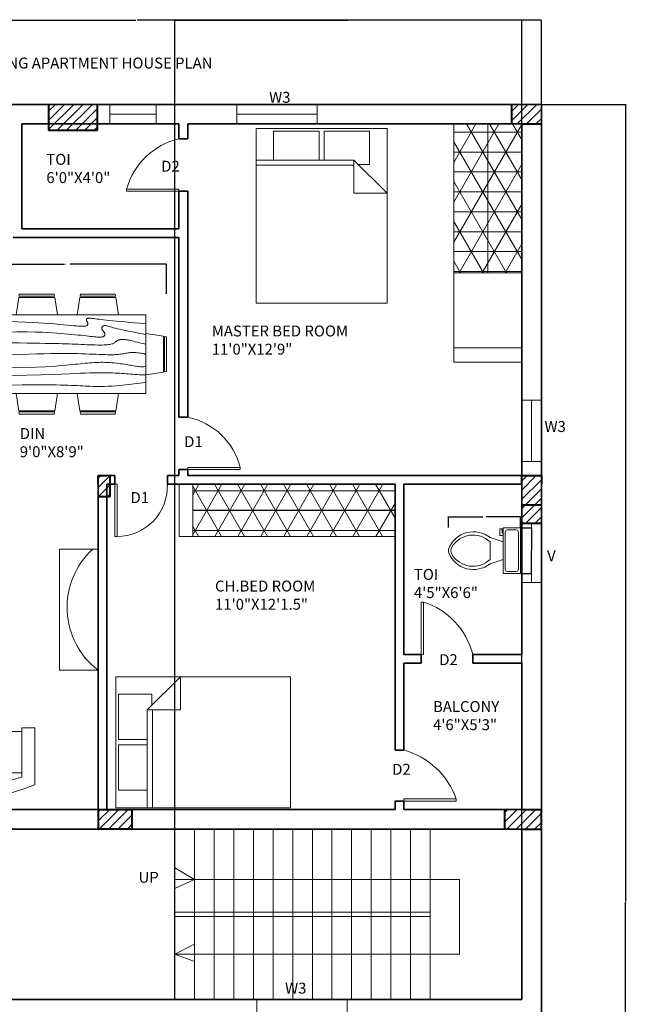
# Model space of a CAD drawing. Units: inches. Extents: x -86 to 2463, y -1058 to 68.
# Tile 17 of 17: x 148 to 426, y -383 to 68. Entities that reach past the tile are written whole.
import ezdxf

# ---------------------------------------------------------------- set-up
doc = ezdxf.new("R2010")
doc.units = ezdxf.units.IN
doc.header["$MEASUREMENT"] = 0
for name, color, linetype, lineweight in [('A-ANNO-DIMS', 2, 'Continuous', 18), ('A-ANNO-TEXT', 7, 'Continuous', 18), ('A-ANNO-TITL', 7, 'Continuous', 25), ('A-AREA-IDEN', 7, 'Continuous', 18), ('A-COLS', 7, 'Continuous', 40), ('A-COLS-PATT', 252, 'Continuous', 13), ('A-DOOR', 3, 'Continuous', 18), ('A-FLOR-CASE', 8, 'Continuous', 18), ('A-FLOR-CASE-PATT', 252, 'Continuous', 13), ('A-FLOR-FIXT', 9, 'Continuous', 18), ('A-FLOR-STRS', 7, 'Continuous', 18), ('A-FURN', 8, 'Continuous', 18), ('A-GLAZ', 4, 'Continuous', 18), ('A-WALL', 7, 'Continuous', 35)]:
    doc.layers.add(name, color=color, linetype=linetype, lineweight=lineweight)
doc.styles.get("Standard").update_dxf_attribs({"font": 'arial.ttf'})
doc.dimstyles.get("Standard").update_dxf_attribs({"dimtxt": 0.18, "dimasz": 0.18, "dimexe": 0.18, "dimexo": 0.0625, "dimgap": 0.09, "dimtad": 0, "dimtih": 1, "dimtoh": 1, "dimdec": 4, "dimzin": 0, "dimdsep": 46, "dimtxsty": 'Standard', "dimcen": 0.09, "dimadec": 0, "dimazin": 0, "dimtfac": 1, "dimtdec": 4, "dimtofl": 0, "dimtmove": 0, "dimatfit": 3, "dimfxl": 1, "dimtolj": 1, "dimtzin": 0, "dimarcsym": 0})
pattern_1 = [(45, (-1015.1314, -586.0864), (-2.1213203, 2.1213203), [])]
pattern_2 = [(0, (-1015.131, -586.086), (0, 9.125), []), (60, (-1015.131, -586.086), (-7.90248, 4.5625), []), (120, (-1015.131, -586.086), (-7.90248, -4.5625), [])]

# ---------------------------------------------------------------- blocks, each defined once
blk = doc.blocks.new('Bed - Queen')
for p, q in [((0, -80.00003), (0, 0)), ((0, 0), (59.99999, 0)), ((59.99999, 0), (59.99999, -80.00003)), ((7.99999, -1.2), (28.79998, -1.2)), ((7.99999, -14.4), (7.99999, -1.2)), ((28.79998, -1.2), (28.79998, -14.4)), ((31.19999, -1.2), (51.99999, -1.2)), ((31.19999, -14.4), (31.19999, -1.2)), ((51.99999, -1.2), (51.99999, -16.4)), ((0, -14.4), (44.8, -14.4)), ((44.8, -16.8), (0, -16.8)), ((59.99999, -29.6), (44.8, -14.4)), ((44.8, -14.4), (44.8, -29.6)), ((51.99999, -16.4), (46.79936, -16.4)), ((44.8, -29.6), (59.99999, -29.6)), ((59.99999, -80.00003), (0, -80.00003))]:
    blk.add_line(p, q)
blk = doc.blocks.new('Toilet - top')
for p, q in [((9.5, -6), (9.5, -2)), ((-10, -8.5), (-8, -8.5)), ((-10, -9.5), (-10, -8.5)), ((-8, -8.5), (-8, -8)), ((-7, -8), (-7, -9.5)), ((-4, -8), (-6, -14)), ((4, -8), (6, -14)), ((-7, -9.5), (-10, -9.5)), ((4, -14), (-4, -14))]:
    blk.add_line(p, q)
blk.add_lwpolyline([(10.5, -8), (10.5, 0), (-10.5, 0), (-10.5, -8)], close=True)
for points in [[(-9.5, -2), (-9.5, -6)], [(8.5, -1), (-8.5, -1)], [(-8.5, -7), (8.5, -7)]]:
    blk.add_lwpolyline(points)
for centre, radius, start, end in [((-8.62, -1.88), 0.884, 81.8699, 188.1301), ((8.62, -1.88), 0.884, 351.8699, 98.1301), ((-8.62, -6.12), 0.884, 171.8699, 278.1301), ((8.62, -6.12), 0.884, 261.8699, 8.1301), ((3.52, -21.58), 12.17, 141.4691, 247.9714), ((4.2, -21.82), 11.33, 136.3677, 238.9468), ((-3.52, -21.58), 12.17, 292.0284, 38.5307), ((-4.2, -21.82), 11.33, 301.053, 43.6321), ((0, -27.88), 4, 245.7318, 294.2682), ((0, -29), 4, 254.8605, 285.1395)]:
    blk.add_arc(centre, radius, start, end)
blk = doc.blocks.new('Sofa - Roundback 7 ft.')
for p, q in [((-12.00002, -32.4421), (-12.00003, -6.5971)), ((11.99997, -32.4421), (11.99998, -6.5971)), ((-36.000027, -34), (-36.000027, -11.4696)), ((-35.999844, -13.3819), (35.9998, -13.3819)), ((35.99998, -34), (35.99998, -11.4696)), ((-36.000027, -32.4421), (35.99998, -32.4421))]:
    blk.add_line(p, q)
for points in [[(-36.000027, -34), (-42.000027, -34), (-42.000027, -8)], [(41.99998, -8), (41.99998, -34), (35.99998, -34)]]:
    blk.add_lwpolyline(points)
for centre, radius, start, end in [((0, -114.25), 114.25, 68.43141, 111.5686), ((-0.00001, -127.1968), 121.1968, 72.72033, 107.2797)]:
    blk.add_arc(centre, radius, start, end)
blk = doc.blocks.new('Dining Set - 36 x 72 in.')
for p, q in [((-22, 27.5), (-22.1562, 26.50042)), ((-22, 27.5), (-6, 27.5)), ((-5.8437, 26.49966), (-6, 27.5)), ((6, 27.5), (5.8438, 26.50042)), ((6, 27.5), (22, 27.5)), ((22.1563, 26.49966), (22, 27.5)), ((-22.2343, 26.00059), (-23.4847, 17.99762)), ((-22.2304, 26), (-5.7608, 26)), ((-5.8416, 26.5), (-22.1534, 26.5)), ((-4.5152, 17.99762), (-5.7655, 25.99926)), ((5.7657, 26.00059), (4.5153, 17.99762)), ((5.7696, 26), (22.2392, 26)), ((22.1584, 26.5), (5.8466, 26.5)), ((23.4848, 17.99762), (22.2345, 25.99926)), ((36, 18), (-36, 18)), ((-36, 18), (-36, -18)), ((36, -18), (36, 18)), ((-44.0006, 8.23428), (-35.9976, 9.48474)), ((44.0006, 8.23428), (35.9976, 9.48474)), ((-45.5, 8), (-44.5004, 8.15617)), ((-45.5, 8), (-45.5, -8)), ((-44.5, -8.15843), (-44.5, 8.15338)), ((-44, 8.23041), (-44, -8.23915)), ((44, 8.23041), (44, -8.23915)), ((44.5, -8.15843), (44.5, 8.15338)), ((45.5, 8), (44.5005, 8.15617)), ((45.5, 8), (45.5, -8)), ((-44.4997, -8.15631), (-45.5, -8)), ((-35.9976, -9.48476), (-43.9993, -8.2345)), ((35.9976, -9.48476), (43.9993, -8.2345)), ((44.4997, -8.15631), (45.5, -8)), ((-36, -18), (36, -18)), ((-22.2343, -26.0006), (-23.4847, -17.99762)), ((-4.5152, -17.99762), (-5.7655, -25.99928)), ((5.7657, -26.0006), (4.5153, -17.99762)), ((23.4848, -17.99762), (22.2345, -25.99928)), ((-22.2304, -26), (-5.7608, -26)), ((-22, -27.5), (-22.1562, -26.50044)), ((-5.8416, -26.5), (-22.1534, -26.5)), ((-5.8437, -26.49967), (-6, -27.5)), ((5.7696, -26), (22.2392, -26)), ((6, -27.5), (5.8438, -26.50044)), ((22.1584, -26.5), (5.8466, -26.5)), ((22.1563, -26.49967), (22, -27.5)), ((-22, -27.5), (-6, -27.5)), ((6, -27.5), (22, -27.5))]:
    blk.add_line(p, q)
for points in [[(-36, 15), (-31.1772, 14.97754), (-26.8079, 14.91406), (-22.8538, 14.81543), (-19.276, 14.6875), (-16.0362, 14.53613), (-13.0957, 14.36718), (-10.4159, 14.18652), (-7.9583, 14), (-5.6904, 13.81315), (-3.6035, 13.63021), (-1.6954, 13.45508), (0.0365, 13.29166), (1.5945, 13.14388), (2.9811, 13.01562), (4.1988, 12.9108), (5.25, 12.83333), (6.1393, 12.78613), (6.8802, 12.76823), (7.4883, 12.77767), (7.9792, 12.8125), (8.3685, 12.87077), (8.6719, 12.95052), (8.9049, 13.0498), (9.0833, 13.16666), (9.2205, 13.29899), (9.3216, 13.44401), (9.3895, 13.59879), (9.4271, 13.76041), (9.4373, 13.92594), (9.4232, 14.09245), (9.3875, 14.257), (9.3333, 14.41666), (9.2638, 14.56917), (9.1836, 14.71484), (9.0975, 14.85465), (9.0104, 14.98958), (8.9272, 15.1206), (8.8529, 15.2487), (8.7922, 15.37483), (8.75, 15.5), (8.7305, 15.62467), (8.7344, 15.74739), (8.7617, 15.86621), (8.8125, 15.97916), (8.8867, 16.08431), (8.9844, 16.17968), (9.1055, 16.26334), (9.25, 16.33333), (9.4189, 16.38802), (9.6172, 16.42708), (9.8506, 16.45052), (10.125, 16.45833), (10.4463, 16.45052), (10.8203, 16.42708), (11.2529, 16.38802), (11.75, 16.33333), (12.3184, 16.26318), (12.9694, 16.17838), (13.7151, 16.07991), (14.5677, 15.96875), (15.5395, 15.84586), (16.6426, 15.71224), (17.8893, 15.56884), (19.2917, 15.41666), (20.859, 15.25667), (22.5879, 15.08984), (24.4721, 14.91715), (26.5052, 14.73958), (28.6809, 14.5581), (30.9929, 14.3737), (33.4347, 14.18733), (36, 14)], [(-36, 10), (-28.9766, 10.14274), (-23.1725, 10.20442), (-18.4241, 10.19775), (-14.5677, 10.13541), (-11.4399, 10.03011), (-8.877, 9.89453), (-6.7154, 9.74137), (-4.7917, 9.58333), (-2.9698, 9.43082), (-1.2246, 9.28515), (0.4415, 9.14534), (2.026, 9.01041), (3.5266, 8.87939), (4.9408, 8.7513), (6.266, 8.62516), (7.5, 8.5), (8.6411, 8.37549), (9.6914, 8.2539), (10.6538, 8.13818), (11.5312, 8.03125), (12.3267, 7.93603), (13.043, 7.85547), (13.6831, 7.79248), (14.25, 7.75), (14.7471, 7.7303), (15.1797, 7.73307), (15.5537, 7.75732), (15.875, 7.80208), (16.1494, 7.86637), (16.3828, 7.94922), (16.5811, 8.04964), (16.75, 8.16666), (16.8944, 8.29915), (17.0143, 8.44531), (17.1089, 8.60319), (17.1771, 8.77083), (17.218, 8.94629), (17.2305, 9.1276), (17.2137, 9.31282), (17.1667, 9.5), (17.0895, 9.6875), (16.987, 9.875), (16.8649, 10.0625), (16.7292, 10.25), (16.5856, 10.4375), (16.4401, 10.625), (16.2985, 10.8125), (16.1667, 11), (16.05, 11.18733), (15.9518, 11.3737), (15.8752, 11.5581), (15.8229, 11.73958), (15.798, 11.91715), (15.8034, 12.08984), (15.842, 12.25667), (15.9167, 12.41666), (16.0295, 12.56836), (16.1784, 12.70833), (16.3605, 12.83268), (16.5729, 12.9375), (16.8127, 13.01888), (17.0768, 13.07291), (17.3625, 13.0957), (17.6667, 13.08333), (17.9894, 13.03312), (18.3418, 12.94726), (18.7382, 12.82918), (19.1927, 12.68229), (19.7195, 12.51001), (20.3327, 12.31575), (21.0465, 12.10294), (21.875, 11.875), (22.8357, 11.63354), (23.959, 11.37304), (25.2786, 11.08618), (26.8282, 10.76562), (28.6414, 10.40405), (30.752, 9.99414), (33.1936, 9.52856), (36, 9)], [(-36, 5.5), (-30.7157, 5.3348), (-26.069, 5.20963), (-21.9946, 5.11767), (-18.4271, 5.05208), (-15.3009, 5.00602), (-12.5508, 4.97265), (-10.1112, 4.94515), (-7.9167, 4.91666), (-5.909, 4.88167), (-4.0586, 4.83984), (-2.3429, 4.79215), (-0.7396, 4.73958), (0.7739, 4.6831), (2.22, 4.6237), (3.6213, 4.56233), (5, 4.5), (6.373, 4.43782), (7.7344, 4.3776), (9.0723, 4.32129), (10.375, 4.27083), (11.6309, 4.22819), (12.8281, 4.19531), (13.9551, 4.17415), (15, 4.16666), (15.954, 4.17448), (16.819, 4.19791), (17.6001, 4.23698), (18.3021, 4.29166), (18.9299, 4.36198), (19.4883, 4.44791), (19.9823, 4.54948), (20.4167, 4.66666), (20.7969, 4.79899), (21.1302, 4.94401), (21.4245, 5.09879), (21.6875, 5.26041), (21.9271, 5.42594), (22.1511, 5.59245), (22.3672, 5.757), (22.5834, 5.91666), (22.8065, 6.06868), (23.0404, 6.21093), (23.2879, 6.34147), (23.5521, 6.45833), (23.8358, 6.55957), (24.142, 6.64323), (24.4735, 6.70735), (24.8334, 6.75), (25.2235, 6.76969), (25.642, 6.76692), (26.0858, 6.74267), (26.5521, 6.69791), (27.0379, 6.63362), (27.5404, 6.55078), (28.0565, 6.45036), (28.5834, 6.33333), (29.1242, 6.19987), (29.7071, 6.04687), (30.3661, 5.87044), (31.1354, 5.66666), (32.0493, 5.43164), (33.142, 5.16146), (34.4475, 4.85221), (36, 4.5)], [(-36, -1), (-30.7915, -0.6591), (-26.0195, -0.38216), (-21.6519, -0.16284), (-17.6563, 0.00521), (-14.0005, 0.12833), (-10.6523, 0.21289), (-7.5796, 0.26522), (-4.75, 0.29166), (-2.134, 0.29793), (0.2878, 0.28711), (2.5317, 0.26163), (4.6146, 0.22396), (6.5529, 0.17651), (8.3633, 0.12174), (10.0623, 0.06209), (11.6667, 0), (13.1899, -0.06201), (14.6341, -0.1211), (15.9982, -0.17432), (17.2813, -0.21875), (18.4823, -0.25147), (19.6003, -0.26953), (20.6343, -0.27002), (21.5834, -0.25), (22.4481, -0.20768), (23.2357, -0.14584), (23.9549, -0.06836), (24.6146, 0.02083), (25.2235, 0.11784), (25.7904, 0.21875), (26.3241, 0.31966), (26.8334, 0.41666), (27.3265, 0.50618), (27.8099, 0.58593), (28.2894, 0.65397), (28.7709, 0.70833), (29.2601, 0.74707), (29.763, 0.76823), (30.2855, 0.76985), (30.8334, 0.75), (31.4088, 0.70784), (31.9994, 0.64713), (32.589, 0.57275), (33.1615, 0.48958), (33.7008, 0.4025), (34.1908, 0.3164), (34.6153, 0.23616), (34.9584, 0.16666), (35.2099, 0.11165), (35.3848, 0.07031), (35.504, 0.04069), (35.5886, 0.02083), (35.6594, 0.00879), (35.7377, 0.0026), (35.8442, 0.00032), (36, 0)], [(-36, -6.5), (-27.1843, -6.31267), (-20.084, -6.1263), (-14.469, -5.9419), (-10.1094, -5.76042), (-6.7752, -5.58285), (-4.2363, -5.41016), (-2.2629, -5.24333), (-0.625, -5.08334), (0.8708, -4.93099), (2.2715, -4.78646), (3.5872, -4.64974), (4.8281, -4.52084), (6.0046, -4.39974), (7.127, -4.28646), (8.2053, -4.18099), (9.25, -4.08334), (10.2705, -3.99382), (11.2734, -3.91407), (12.2647, -3.84603), (13.25, -3.79167), (14.2354, -3.75293), (15.2266, -3.73177), (16.2295, -3.73015), (17.25, -3.75), (18.2912, -3.79248), (19.3451, -3.85547), (20.4009, -3.93604), (21.4479, -4.03125), (22.4754, -4.13819), (23.4727, -4.25391), (24.4289, -4.37549), (25.3334, -4.5), (26.1785, -4.62492), (26.9694, -4.74935), (27.7145, -4.87281), (28.4219, -4.99479), (29.1, -5.11483), (29.7572, -5.23242), (30.4016, -5.34709), (31.0417, -5.45834), (31.6837, -5.56437), (32.3262, -5.65821), (32.9658, -5.73153), (33.599, -5.77604), (34.2224, -5.78345), (34.8327, -5.74545), (35.4264, -5.65373), (36, -5.5)], [(-36, -10), (-26.4022, -9.81299), (-18.4675, -9.62891), (-11.9839, -9.45069), (-6.7396, -9.28125), (-2.5226, -9.12354), (0.8789, -8.98047), (3.6769, -8.85498), (6.0833, -8.75), (8.2767, -8.66765), (10.3021, -8.60677), (12.1712, -8.56543), (13.8958, -8.54167), (15.4876, -8.53353), (16.9583, -8.53907), (18.3197, -8.55632), (19.5834, -8.58334), (20.7616, -8.61841), (21.8685, -8.66081), (22.9188, -8.71004), (23.9271, -8.76563), (24.9081, -8.82707), (25.8763, -8.89388), (26.8465, -8.96558), (27.8334, -9.04167), (28.8474, -9.12118), (29.8828, -9.20117), (30.93, -9.27824), (31.9792, -9.34896), (33.0205, -9.40991), (34.0443, -9.45768), (35.0407, -9.48885), (36, -9.5)], [(-36, -14.5), (-30.0881, -14.33513), (-25.0332, -14.21224), (-20.7312, -14.12647), (-17.0781, -14.07292), (-13.97, -14.04671), (-11.3027, -14.04297), (-8.9724, -14.05681), (-6.875, -14.08334), (-4.9224, -14.11833), (-3.0905, -14.16016), (-1.3709, -14.20785), (0.2448, -14.26042), (1.7647, -14.3169), (3.1973, -14.3763), (4.5507, -14.43767), (5.8333, -14.5), (7.0554, -14.5621), (8.235, -14.62175), (9.3922, -14.67652), (10.5469, -14.72396), (11.7192, -14.76164), (12.929, -14.78711), (14.1965, -14.79794), (15.5417, -14.79167), (16.9933, -14.76424), (18.6152, -14.70508), (20.4804, -14.60197), (22.6615, -14.44271), (25.2312, -14.21509), (28.2624, -13.9069), (31.8277, -13.50594), (36, -13)]]:
    blk.add_lwpolyline(points)
blk = doc.blocks.new('DOOR-LEAF-24IN')
for p, q in [((0, 0), (0, 24)), ((0, 24), (1, 24)), ((1, 24), (1, 0)), ((1, 0), (0, 0))]:
    blk.add_line(p, q)
blk = doc.blocks.new('*D22')
at = {"layer": 'A-ANNO-DIMS', "color": 0, "lineweight": -2, "transparency": 16777216}
for p, q in [((344.18, -164.99), (344.18, -159.92)), ((344.36, -160.1), (359.93, -160.1)), ((377.05, -160.1), (361.48, -160.1)), ((377.23, -164.99), (377.23, -159.92))]:
    blk.add_line(p, q, dxfattribs=at)
at = {"layer": 'A-ANNO-DIMS', "color": 0, "transparency": 16777216}
for points in [[(344.36, -160.07), (344.36, -160.13), (344.18, -160.1)], [(377.05, -160.07), (377.05, -160.13), (377.23, -160.1)]]:
    blk.add_solid(points, dxfattribs=at)
at = {"layer": 'Defpoints', "color": 0, "transparency": 16777216}
for p in [(377.23, -160.1), (344.18, -165.05), (377.23, -165.05)]:
    blk.add_point(p, dxfattribs=at)
at = {"layer": 'A-ANNO-DIMS', "color": 0, "transparency": 16777216, "insert": (360.71, -160.1), "char_height": 0.18, "attachment_point": 5}
blk.add_mtext('\\A1;WC 33 TYP.', dxfattribs=at)
blk = doc.blocks.new('*D23')
at = {"layer": 'A-ANNO-DIMS', "color": 0, "lineweight": -2, "transparency": 16777216}
for p, q in [((377.29, -165.05), (382.37, -165.05)), ((382.19, -165.23), (382.19, -175.37)), ((382.19, -185.87), (382.19, -175.73)), ((377.29, -186.05), (382.37, -186.05))]:
    blk.add_line(p, q, dxfattribs=at)
at = {"layer": 'A-ANNO-DIMS', "color": 0, "transparency": 16777216}
for points in [[(382.16, -165.23), (382.22, -165.23), (382.19, -165.05)], [(382.16, -185.87), (382.22, -185.87), (382.19, -186.05)]]:
    blk.add_solid(points, dxfattribs=at)
at = {"layer": 'Defpoints', "color": 0, "transparency": 16777216}
for p in [(377.23, -165.05), (377.23, -186.05), (382.19, -186.05)]:
    blk.add_point(p, dxfattribs=at)
at = {"layer": 'A-ANNO-DIMS', "color": 0, "transparency": 16777216, "insert": (382.19, -175.55), "char_height": 0.18, "attachment_point": 5}
blk.add_mtext('\\A1;21 TYP.', dxfattribs=at)
blk = doc.blocks.new('*D28')
at = {"layer": 'A-ANNO-DIMS', "color": 0, "lineweight": -2, "transparency": 16777216}
for p, q in [((124.1, -57.97), (124.1, -44.2)), ((124.28, -44.38), (168.32, -44.38)), ((214.92, -44.38), (170.87, -44.38)), ((215.1, -57.97), (215.1, -44.2))]:
    blk.add_line(p, q, dxfattribs=at)
at = {"layer": 'A-ANNO-DIMS', "color": 0, "transparency": 16777216}
for points in [[(124.28, -44.35), (124.28, -44.41), (124.1, -44.38)], [(214.92, -44.35), (214.92, -44.41), (215.1, -44.38)]]:
    blk.add_solid(points, dxfattribs=at)
at = {"layer": 'Defpoints', "color": 0, "transparency": 16777216}
for p in [(215.1, -44.38), (124.1, -58.03), (215.1, -58.03)]:
    blk.add_point(p, dxfattribs=at)
at = {"layer": 'A-ANNO-DIMS', "color": 0, "transparency": 16777216, "insert": (169.6, -44.38), "char_height": 0.18, "attachment_point": 5}
blk.add_mtext('\\A1;DINING SET 91 TYP.', dxfattribs=at)
blk = doc.blocks.new('*D31')
at = {"layer": 'A-ANNO-DIMS', "color": 0, "lineweight": -2, "transparency": 16777216}
for p, q in [((386.82, 28.9), (425.54, 28.9)), ((425.36, 28.72), (425.36, -336.17)), ((425.36, -701.42), (425.36, -336.54)), ((386.82, -701.6), (425.54, -701.6))]:
    blk.add_line(p, q, dxfattribs=at)
at = {"layer": 'A-ANNO-DIMS', "color": 0, "transparency": 16777216}
for points in [[(425.33, 28.72), (425.39, 28.72), (425.36, 28.9)], [(425.33, -701.42), (425.39, -701.42), (425.36, -701.6)]]:
    blk.add_solid(points, dxfattribs=at)
at = {"layer": 'Defpoints', "color": 0, "transparency": 16777216}
for p in [(386.76, 28.9), (425.36, 28.9), (386.76, -701.6)]:
    blk.add_point(p, dxfattribs=at)
at = {"layer": 'A-ANNO-DIMS', "color": 0, "transparency": 16777216, "insert": (425.36, -336.35), "char_height": 0.18, "attachment_point": 5}
blk.add_mtext('\\A1;730.5', dxfattribs=at)
blk = doc.blocks.new('*D35')
at = {"layer": 'A-ANNO-DIMS', "color": 0, "lineweight": -2, "transparency": 16777216}
for p, q in [((15.76, 28.96), (15.76, 67.68)), ((386.76, 28.96), (386.76, 67.68)), ((15.94, 67.5), (200.99, 67.5)), ((386.58, 67.5), (201.53, 67.5))]:
    blk.add_line(p, q, dxfattribs=at)
at = {"layer": 'A-ANNO-DIMS', "color": 0, "transparency": 16777216}
for points in [[(15.94, 67.53), (15.94, 67.47), (15.76, 67.5)], [(386.58, 67.53), (386.58, 67.47), (386.76, 67.5)]]:
    blk.add_solid(points, dxfattribs=at)
at = {"layer": 'Defpoints', "color": 0, "transparency": 16777216}
for p in [(386.76, 67.5), (15.76, 28.9), (386.76, 28.9)]:
    blk.add_point(p, dxfattribs=at)
at = {"layer": 'A-ANNO-DIMS', "color": 0, "transparency": 16777216, "insert": (201.26, 67.5), "char_height": 0.18, "attachment_point": 5}
blk.add_mtext('\\A1;371', dxfattribs=at)
blk = doc.blocks.new('*D36')
at = {"layer": 'A-ANNO-DIMS', "color": 0, "lineweight": -2, "transparency": 16777216}
for p, q in [((218.85, -381.04), (218.85, 67.68)), ((377.85, -381.04), (377.85, 67.68)), ((219.03, 67.5), (298.07, 67.5)), ((377.67, 67.5), (298.63, 67.5))]:
    blk.add_line(p, q, dxfattribs=at)
at = {"layer": 'A-ANNO-DIMS', "color": 0, "transparency": 16777216}
for points in [[(219.03, 67.53), (219.03, 67.47), (218.85, 67.5)], [(377.67, 67.53), (377.67, 67.47), (377.85, 67.5)]]:
    blk.add_solid(points, dxfattribs=at)
at = {"layer": 'Defpoints', "color": 0, "transparency": 16777216}
for p in [(377.85, 67.5), (218.85, -381.1), (377.85, -381.1)]:
    blk.add_point(p, dxfattribs=at)
at = {"layer": 'A-ANNO-DIMS', "color": 0, "transparency": 16777216, "insert": (298.35, 67.5), "char_height": 0.18, "attachment_point": 5}
blk.add_mtext('\\A1;159', dxfattribs=at)

msp = doc.modelspace()

# ---------------------------------------------------------------- hatches: boundary and pattern name
at = {"layer": 'A-COLS-PATT'}
h = msp.add_hatch(dxfattribs=at)
h.set_pattern_fill('ANSI31', color=256, scale=24)
h.set_pattern_definition(pattern_1)
h.paths.add_polyline_path([(24.761, -294.104), (24.761, -284.978), (15.761, -284.978), (15.761, -303.104), (24.761, -303.104)])
h.paths.add_polyline_path([(199.1, -294.104), (183.761, -294.104), (183.761, -303.104), (199.1, -303.104)])
h.paths.add_polyline_path([(386.761, -294.104), (377.761, -294.104), (369.914, -294.104), (369.914, -303.104), (377.846, -303.104), (386.761, -303.104)])
h.paths.add_polyline_path([(386.761, -145.104), (386.761, -141.104), (377.761, -141.104), (377.761, -145.104), (377.761, -154.61), (386.761, -154.61)])
h.paths.add_polyline_path([(386.761, -154.61), (377.761, -154.61), (377.761, -162.891), (386.761, -162.891)])
h.paths.add_polyline_path([(24.761, -145.104), (24.761, -141.104), (15.761, -141.104), (15.761, -156.678), (24.761, -156.678)])
h.paths.add_polyline_path([(-38.239, 28.896), (-47.239, 28.896), (-47.239, 19.896), (-47.239, 12.652), (-38.239, 12.652), (-38.239, 19.896)])
h.paths.add_polyline_path([(24.761, 28.896), (15.761, 28.896), (15.761, 19.896), (15.761, 12.545), (24.761, 12.545), (24.761, 19.896)])
h.paths.add_polyline_path([(183.507, 19.896), (161.036, 19.896), (161.036, 17.001), (183.507, 17.001)])
h.paths.add_polyline_path([(183.507, 28.896), (161.036, 28.896), (161.036, 19.896), (183.507, 19.896)])
h.paths.add_polyline_path([(386.761, 28.896), (373.166, 28.896), (373.166, 19.896), (377.761, 19.896), (386.761, 19.896)])
h = msp.add_hatch(dxfattribs=at)
h.set_pattern_fill('ANSI31', color=256, scale=24)
h.set_pattern_definition(pattern_1)
h.paths.add_polyline_path([(189.136, -141.104), (187.761, -141.104), (183.761, -141.104), (183.761, -145.104), (183.761, -150.833), (187.761, -150.833), (187.761, -145.104), (189.136, -145.104)])
h.paths.add_polyline_path([(189.136, -145.104), (187.761, -145.104), (187.761, -150.833), (189.136, -150.833)], flags=17)
at = {"layer": 'A-FLOR-CASE-PATT'}
h = msp.add_hatch(dxfattribs=at)
h.set_pattern_fill('NET3', color=256, scale=73)
h.set_pattern_definition(pattern_2)
h.paths.add_polyline_path([(362.202, 19.896), (346.643, 19.896), (346.643, -48.262), (362.202, -48.262)])
h.paths.add_polyline_path([(377.761, 19.896), (362.202, 19.896), (362.202, -48.262), (377.761, -48.262)])
h.paths.add_polyline_path([(362.455, -390.104), (347.604, -390.104), (347.604, -460.245), (362.455, -460.245)])
h.paths.add_polyline_path([(377.846, -390.104), (362.455, -390.104), (362.455, -460.245), (377.846, -460.245), (377.846, -425.104), (377.846, -421.104)])
h = msp.add_hatch(dxfattribs=at)
h.set_pattern_fill('NET3', color=256, scale=73)
h.set_pattern_definition(pattern_2)
h.paths.add_polyline_path([(319.761, -145.104), (227.044, -145.104), (227.044, -157.07), (319.761, -157.07)])
h.paths.add_polyline_path([(319.761, -157.07), (227.044, -157.07), (227.044, -169.036), (319.761, -169.036)])
h.paths.add_polyline_path([(319.846, -547.104), (234.906, -547.104), (234.906, -563.554), (319.846, -563.554)])
h.paths.add_polyline_path([(319.846, -563.554), (234.906, -563.554), (234.906, -580.004), (319.846, -580.004)])

# ---------------------------------------------------------------- linework, layer by layer
at = {"layer": 'A-COLS'}
for p, q in [((161.036, 28.896), (161.036, 17.001)), ((183.507, 17.001), (183.507, 28.896)), ((373.166, 19.896), (373.166, 28.896)), ((377.761, 19.896), (386.761, 19.896)), ((161.036, 17.001), (183.507, 17.001)), ((183.761, -141.104), (187.761, -141.104)), ((183.761, -145.104), (183.761, -141.104)), ((189.136, -141.104), (189.136, -150.833)), ((377.761, -141.104), (386.761, -141.104)), ((377.761, -145.104), (377.761, -141.104)), ((386.761, -141.104), (386.761, -145.104)), ((189.136, -150.833), (183.761, -150.833)), ((377.761, -154.61), (386.761, -154.61)), ((377.761, -162.891), (386.761, -162.891)), ((183.761, -294.104), (199.1, -294.104)), ((183.761, -294.104), (183.761, -303.104)), ((199.1, -294.104), (199.1, -303.104)), ((369.914, -294.104), (369.914, -303.104)), ((377.761, -294.104), (386.761, -294.104)), ((386.761, -303.104), (386.761, -294.104)), ((199.1, -303.104), (183.488, -303.104)), ((377.846, -303.104), (386.761, -303.104))]:
    msp.add_line(p, q, dxfattribs=at)
at = {"layer": 'A-DOOR'}
msp.add_line((220.761, -9.914), (220.761, -9.914), dxfattribs=at)
for centre, radius, start, end in [((228.021, -18.512), 32.421, 102.9403, 164.62195), ((218.621, -144.874), 31.041, 13.84523, 78.59252), ((192.286, -145.928), 23.177, 270.40058, 2.03717), ((322.741, -231.116), 33.53, 13.82397, 72.69243), ((314.756, -300.701), 34.927, 19.09458, 75.05907)]:
    msp.add_arc(centre, radius, start, end, dxfattribs=at)
at = {"layer": 'A-FLOR-CASE'}
for p, q in [((346.643, -89.261), (346.643, 19.896)), ((362.202, -48.262), (362.202, 19.896)), ((346.643, -48.262), (377.761, -48.262)), ((346.643, -82.695), (377.761, -82.695)), ((377.761, -89.261), (346.643, -89.261)), ((220.887, -145.104), (220.887, -169.036)), ((227.044, -145.104), (227.044, -169.036)), ((227.044, -157.07), (319.761, -157.07)), ((220.887, -169.036), (319.761, -169.036)), ((183.761, -174.88), (166.035, -174.88)), ((166.035, -174.88), (166.035, -230.353)), ((166.035, -230.353), (183.761, -230.353))]:
    msp.add_line(p, q, dxfattribs=at)
msp.add_arc((205.679, -201.556), 36.189, 132.51187, 232.72477, dxfattribs=at)
at = {"layer": 'A-FLOR-STRS'}
for p, q in [((218.852, -303.104), (218.852, -381.104)), ((227.852, -303.104), (227.852, -381.104)), ((236.852, -303.104), (236.852, -381.104)), ((245.852, -303.104), (245.852, -381.104)), ((254.852, -303.104), (254.852, -381.104)), ((263.852, -303.104), (263.852, -381.104)), ((272.852, -303.104), (272.852, -381.104)), ((281.852, -303.104), (281.852, -381.104)), ((290.852, -303.104), (290.852, -381.104)), ((299.852, -303.104), (299.852, -381.104)), ((308.852, -303.104), (308.852, -381.104)), ((317.852, -303.104), (317.852, -381.104)), ((326.852, -303.104), (326.852, -381.104)), ((335.852, -303.104), (335.852, -381.104)), ((227.852, -326.213), (218.852, -320.879)), ((349.267, -326.213), (218.852, -326.213)), ((227.852, -326.213), (218.852, -330.316)), ((349.267, -360.326), (349.267, -326.213)), ((335.852, -341.104), (218.852, -341.104)), ((335.852, -343.104), (218.852, -343.104)), ((218.852, -360.326), (227.852, -355.759)), ((218.852, -360.326), (349.267, -360.326)), ((218.852, -360.326), (227.852, -363.713))]:
    msp.add_line(p, q, dxfattribs=at)
at = {"layer": 'A-GLAZ'}
for p, q in [((189.065, 19.896), (189.065, 28.896)), ((210.328, 19.896), (210.328, 28.896)), ((247.202, 19.896), (247.202, 28.896)), ((284.008, 28.896), (284.008, 19.896)), ((189.065, 24.396), (210.328, 24.396)), ((247.202, 24.396), (284.008, 24.396)), ((377.761, -106.684), (386.761, -106.684)), ((382.261, -134.737), (382.261, -106.684)), ((377.761, -134.737), (386.761, -134.737)), ((382.261, -162.891), (382.261, -190.097)), ((377.761, -190.097), (386.761, -190.097)), ((256.416, -390.104), (256.416, -381.104)), ((297.782, -390.104), (297.782, -381.104))]:
    msp.add_line(p, q, dxfattribs=at)
at = {"layer": 'A-WALL'}
for p, q in [((124.761, 28.896), (386.761, 28.896)), ((386.761, -143.104), (386.761, 28.896)), ((148.761, -28.104), (148.761, 19.896)), ((148.761, 19.896), (220.761, 19.896)), ((220.761, 13.086), (220.761, 19.896)), ((224.761, 19.896), (377.761, 19.896)), ((224.761, 13.086), (224.761, 19.896)), ((377.761, -141.104), (377.761, 19.896)), ((220.761, 13.086), (224.761, 13.086)), ((220.761, -28.104), (220.761, -10.914)), ((220.761, -10.914), (224.761, -10.914)), ((224.761, -114.445), (224.761, -10.914)), ((148.761, -28.104), (220.761, -28.104)), ((144.761, -32.104), (220.761, -32.104)), ((220.761, -114.445), (220.761, -32.104)), ((220.761, -114.445), (224.761, -114.445)), ((220.761, -141.104), (220.761, -138.445)), ((220.761, -138.445), (224.761, -138.445)), ((224.761, -141.104), (224.761, -138.445)), ((187.761, -141.104), (191.448, -141.104)), ((191.448, -141.104), (191.448, -145.104)), ((215.448, -141.104), (215.448, -145.104)), ((215.448, -141.104), (220.761, -141.104)), ((224.761, -141.104), (377.761, -141.104)), ((183.761, -145.104), (183.761, -294.104)), ((187.761, -145.104), (187.761, -294.104)), ((187.761, -145.104), (191.448, -145.104)), ((215.448, -145.104), (319.761, -145.104)), ((319.761, -145.104), (319.761, -266.955)), ((323.761, -145.104), (323.761, -223.104)), ((323.761, -145.104), (377.761, -145.104)), ((377.761, -145.104), (377.761, -223.104)), ((386.761, -145.104), (386.761, -294.104)), ((323.761, -223.104), (331.716, -223.104)), ((331.716, -223.104), (331.716, -227.104)), ((355.299, -223.104), (355.299, -227.104)), ((355.299, -223.104), (377.761, -223.104)), ((323.761, -227.104), (331.716, -227.104)), ((323.761, -227.104), (323.761, -266.955)), ((355.299, -227.104), (377.761, -227.104)), ((377.761, -227.104), (377.761, -294.104)), ((319.761, -266.955), (323.761, -266.955)), ((319.688, -290.275), (323.761, -290.275)), ((319.761, -290.275), (319.761, -294.104)), ((323.761, -290.275), (323.761, -294.104)), ((183.761, -294.104), (24.761, -294.104)), ((187.761, -294.104), (319.761, -294.104)), ((323.761, -294.104), (377.761, -294.104)), ((377.846, -303.104), (15.761, -303.104)), ((377.846, -303.104), (377.846, -381.104)), ((386.761, -303.104), (386.761, -381.104)), ((377.846, -381.104), (15.761, -381.104)), ((386.761, -390.104), (386.761, -381.104))]:
    msp.add_line(p, q, dxfattribs=at)

# ---------------------------------------------------------------- block references
at = {"layer": 'A-DOOR'}
for p, rotation in [((196.761, -9.914), 270.0000000000001), ((224.761, -137.445), 270.0000000000002), ((192.448, -145.104), 180), ((332.716, -199.104), 180), ((323.761, -289.275), 270.0000000000001)]:
    msp.add_blockref('DOOR-LEAF-24IN', p, dxfattribs=dict(at, rotation=rotation))
at = {"layer": 'A-FLOR-FIXT', "rotation": 270}
msp.add_blockref('Toilet - top', (377.231, -175.553), dxfattribs=at)
at = {"layer": 'A-FURN'}
for name, p in [('Bed - Queen', (256.103, 17.795)), ('Dining Set - 36 x 72 in.', (169.597, -85.531))]:
    msp.add_blockref(name, p, dxfattribs=at)
for name, p, rotation in [('Bed - Queen', (191.859, -293.323), 90), ('Sofa - Roundback 7 ft.', (112.715, -290.771), 180)]:
    msp.add_blockref(name, p, dxfattribs=dict(at, rotation=rotation))

# ---------------------------------------------------------------- texts
at = {"layer": 'A-ANNO-TEXT', "char_height": 5, "attachment_point": 1}
for s, width, insert in [('W3', 20.14781, (262.057, 34.621)), ('D2', 25.39586, (212.619, 3.06)), ('W3', 8.99867, (388.19, -116.199)), ('D1', 12.81448, (223.146, -123.109)), ('D1', 12.81448, (198.574, -148.708)), ('V', 4.19937, (389.388, -175.388)), ('D2', 6.00186, (339.986, -222.994)), ('D2', 7.87745, (318.417, -273.201)), ('UP', 11.21736, (202.239, -322.673)), ('W3', 28.42045, (269.361, -373.466))]:
    msp.add_mtext_dynamic_manual_height_columns(s, width=width, gutter_width=25, heights=[0], dxfattribs=dict(at, insert=insert))
at = {"layer": 'A-ANNO-TITL', "insert": (89.471, 50.312), "char_height": 5, "attachment_point": 1}
msp.add_mtext_dynamic_manual_height_columns('40X60 EAST FACING APARTMENT HOUSE PLAN', width=543.41592, gutter_width=25, heights=[0], dxfattribs=at)
at = {"layer": 'A-AREA-IDEN', "char_height": 5, "attachment_point": 1}
for s, width, insert in [('TOI\\P6\'0"X4\'0"', 24.13948, (159.996, 6.186)), ('MASTER BED ROOM\\P11\'0"X12\'9"', 128.16745, (235.787, -72.422)), ('DIN\\P9\'0"X8\'9"', 33.48911, (147.832, -119.395)), ('TOI\\P4\'5"X6\'6"', 37.88678, (328.375, -183.934)), ('CH.BED ROOM\\P11\'0"X12\'1.5"', 110.29173, (237.274, -189.271)), ('BALCONY\\P4\'6"X5\'3"', 41.28173, (337.145, -244.441))]:
    msp.add_mtext_dynamic_manual_height_columns(s, width=width, gutter_width=25, heights=[0], dxfattribs=dict(at, insert=insert))

# ---------------------------------------------------------------- dimensions: what is measured, and where the dimension line sits
at = {"layer": 'A-ANNO-DIMS'}
for base, p1, p2, picture, middle in [((386.761, 67.496), (15.761, 28.896), (386.761, 28.896), '*D35', (201.261, 67.496)), ((377.846, 67.496), (218.852, -381.104), (377.846, -381.104), '*D36', (298.349, 67.496))]:
    dim = msp.add_linear_dim(base=base, p1=p1, p2=p2, dimstyle='Standard', override={"dimdec": 0, "dimlfac": 1, "dimrnd": 0, "dimzin": 0, "dimdsep": 46, "dimlunit": 2}, dxfattribs=at)
    dim.commit()
    dim.dimension.update_dxf_attribs({"geometry": picture, "text_midpoint": middle})
dim = msp.add_linear_dim(base=(425.361, 28.896), p1=(386.761, -701.604), p2=(386.761, 28.896), angle=90, dimstyle='Standard', override={"dimdec": 1, "dimlfac": 1, "dimrnd": 0, "dimzin": 0, "dimdsep": 46, "dimlunit": 2}, dxfattribs=at)
dim.commit()
dim.dimension.update_dxf_attribs({"geometry": '*D31', "text_midpoint": (425.361, -336.354)})
for base, p1, p2, text, picture, middle in [((215.097, -44.381), (124.097, -58.031), (215.097, -58.031), 'DINING SET <> TYP.', '*D28', (169.597, -44.381)), ((377.231, -160.096), (344.185, -165.053), (377.231, -165.053), 'WC <> TYP.', '*D22', (360.708, -160.096))]:
    dim = msp.add_linear_dim(base=base, p1=p1, p2=p2, text=text, dimstyle='Standard', override={"dimdec": 0, "dimlfac": 1, "dimrnd": 0, "dimzin": 0, "dimdsep": 46, "dimlunit": 2}, dxfattribs=at)
    dim.commit()
    dim.dimension.update_dxf_attribs({"geometry": picture, "text_midpoint": middle})
dim = msp.add_linear_dim(base=(382.188, -186.053), p1=(377.231, -165.053), p2=(377.231, -186.053), angle=270, text='<> TYP.', dimstyle='Standard', override={"dimdec": 0, "dimlfac": 1, "dimrnd": 0, "dimzin": 0, "dimdsep": 46, "dimlunit": 2}, dxfattribs=at)
dim.commit()
dim.dimension.update_dxf_attribs({"geometry": '*D23', "text_midpoint": (382.188, -175.553)})

doc.saveas('drawing.dxf')
